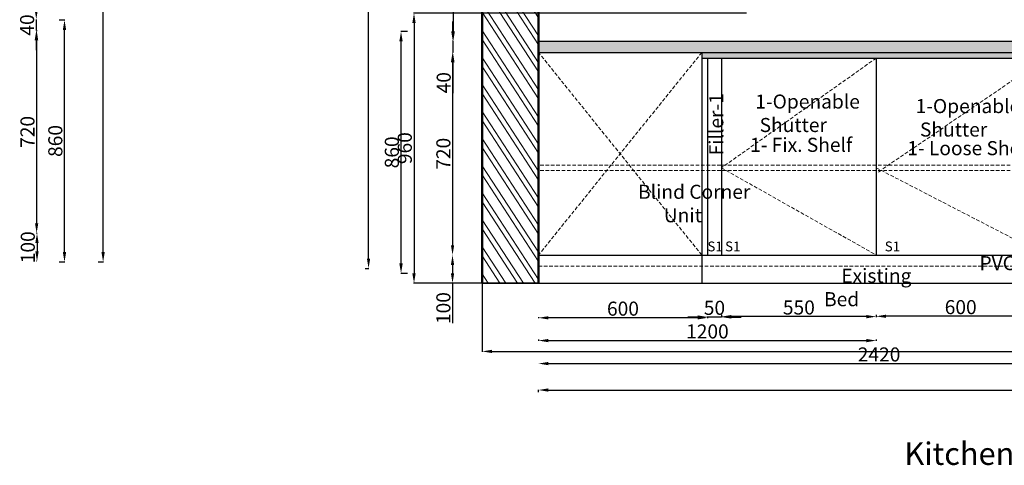
# Model space of a CAD drawing. Units: millimetres. Extents: x 407065 to 421840, y 1168257 to 1177792.
# Tile 15 of 17: x 415758 to 419256, y 1173419 to 1175003. Entities that reach past the tile are written whole.
import ezdxf

# ---------------------------------------------------------------- set-up
doc = ezdxf.new("R2010")
doc.units = ezdxf.units.MM
doc.linetypes.add('DASHED', pattern=[19.05, 12.7, -6.35])
for name, color, linetype, lineweight in [('A-ANNO-DIMS', 6, 'Continuous', 18), ('A-ANNO-TEXT', 30, 'Continuous', 18), ('A-FURN', 3, 'Continuous', 25), ('A-FURN-HIDN', 7, 'DASHED', 18), ('A-FURN-PATT', 252, 'Continuous', 13), ('A-WALL', 7, 'Continuous', 50), ('A-WALL-PATT', 8, 'Continuous', 13)]:
    doc.layers.add(name, color=color, linetype=linetype, lineweight=lineweight)
doc.styles.get("Standard").update_dxf_attribs({"font": 'arial.ttf'})
doc.dimstyles.new('ISO-25', dxfattribs={"dimtxt": 50, "dimasz": 35, "dimexe": 1.25, "dimexo": 0.625, "dimtad": 1, "dimdec": 1, "dimtxsty": 'Standard', "dimcen": 35, "dimadec": 0, "dimazin": 0, "dimtfac": 1, "dimtdec": 1, "dimtmove": 0, "dimatfit": 3, "dimfxl": 1, "dimarcsym": 0})

# ---------------------------------------------------------------- blocks, each defined once
blk = doc.blocks.new('*D67')
at = {"layer": 'A-ANNO-DIMS', "color": 0, "lineweight": -2, "transparency": 16777216}
for p, q in [((415816.7, 1175038.9), (415816.7, 1175073.9)), ((415816.7, 1175003.9), (415816.7, 1174963.9)), ((415817.3, 1175003.9), (415817.9, 1175003.9)), ((415817.3, 1174963.9), (415817.9, 1174963.9)), ((415816.7, 1174928.9), (415816.7, 1174893.9))]:
    blk.add_line(p, q, dxfattribs=at)
at = {"layer": 'A-ANNO-DIMS', "color": 0, "transparency": 16777216}
for points in [[(415810.8, 1175038.9), (415822.5, 1175038.9), (415816.7, 1175003.9)], [(415810.8, 1174928.9), (415822.5, 1174928.9), (415816.7, 1174963.9)]]:
    blk.add_solid(points, dxfattribs=at)
at = {"layer": 'Defpoints', "color": 0, "transparency": 16777216}
for p in [(415816.7, 1175003.9), (415816.7, 1174963.9), (415816.7, 1174963.9)]:
    blk.add_point(p, dxfattribs=at)
at = {"layer": 'A-ANNO-DIMS', "color": 0, "transparency": 16777216, "insert": (415790.5, 1174983.9), "char_height": 50, "attachment_point": 5, "rotation": 90}
blk.add_mtext('40', dxfattribs=at)
blk = doc.blocks.new('*D68')
at = {"layer": 'A-ANNO-DIMS', "color": 0, "lineweight": -2, "transparency": 16777216}
for p, q in [((415817.3, 1174963.9), (415819.2, 1174963.9)), ((415817.9, 1174928.9), (415817.9, 1174278.9)), ((415817.3, 1174243.9), (415819.2, 1174243.9))]:
    blk.add_line(p, q, dxfattribs=at)
at = {"layer": 'A-ANNO-DIMS', "color": 0, "transparency": 16777216}
for points in [[(415812.1, 1174928.9), (415823.7, 1174928.9), (415817.9, 1174963.9)], [(415812.1, 1174278.9), (415823.7, 1174278.9), (415817.9, 1174243.9)]]:
    blk.add_solid(points, dxfattribs=at)
at = {"layer": 'Defpoints', "color": 0, "transparency": 16777216}
for p in [(415816.7, 1174963.9), (415816.7, 1174243.9), (415817.9, 1174243.9)]:
    blk.add_point(p, dxfattribs=at)
at = {"layer": 'A-ANNO-DIMS', "color": 0, "transparency": 16777216, "insert": (415791.8, 1174603.9), "char_height": 50, "attachment_point": 5, "rotation": 90}
blk.add_mtext('720', dxfattribs=at)
blk = doc.blocks.new('*D69')
at = {"layer": 'A-ANNO-DIMS', "color": 0, "lineweight": -2, "transparency": 16777216}
for p, q in [((415818.5, 1174243.9), (415817.9, 1174243.9)), ((415819.2, 1174208.9), (415819.2, 1174178.9)), ((415818.5, 1174143.9), (415817.9, 1174143.9))]:
    blk.add_line(p, q, dxfattribs=at)
at = {"layer": 'A-ANNO-DIMS', "color": 0, "transparency": 16777216}
for points in [[(415813.3, 1174208.9), (415825, 1174208.9), (415819.2, 1174243.9)], [(415813.3, 1174178.9), (415825, 1174178.9), (415819.2, 1174143.9)]]:
    blk.add_solid(points, dxfattribs=at)
at = {"layer": 'Defpoints', "color": 0, "transparency": 16777216}
for p in [(415819.2, 1174243.9), (415819.2, 1174143.9), (415819.2, 1174143.9)]:
    blk.add_point(p, dxfattribs=at)
at = {"layer": 'A-ANNO-DIMS', "color": 0, "transparency": 16777216, "insert": (415793, 1174193.9), "char_height": 50, "attachment_point": 5, "rotation": 90}
blk.add_mtext('100', dxfattribs=at)
blk = doc.blocks.new('*D70')
at = {"layer": 'A-ANNO-DIMS', "color": 0, "lineweight": -2, "transparency": 16777216}
for p, q in [((415898.4, 1175001.7), (415918.2, 1175001.7)), ((415916.9, 1174176.7), (415916.9, 1174966.7)), ((415898.4, 1174141.7), (415918.2, 1174141.7))]:
    blk.add_line(p, q, dxfattribs=at)
at = {"layer": 'A-ANNO-DIMS', "color": 0, "transparency": 16777216}
for points in [[(415911.1, 1174966.7), (415922.8, 1174966.7), (415916.9, 1175001.7)], [(415911.1, 1174176.7), (415922.8, 1174176.7), (415916.9, 1174141.7)]]:
    blk.add_solid(points, dxfattribs=at)
at = {"layer": 'Defpoints', "color": 0, "transparency": 16777216}
for p in [(415897.8, 1175001.7), (415916.9, 1175001.7), (415897.8, 1174141.7)]:
    blk.add_point(p, dxfattribs=at)
at = {"layer": 'A-ANNO-DIMS', "color": 0, "transparency": 16777216, "insert": (415890.8, 1174571.7), "char_height": 50, "attachment_point": 5, "rotation": 90}
blk.add_mtext('860', dxfattribs=at)
blk = doc.blocks.new('*D71')
at = {"layer": 'A-ANNO-DIMS', "color": 0, "lineweight": -2, "transparency": 16777216}
for p, q in [((416036.8, 1176991.7), (416055.3, 1176991.7)), ((416054.1, 1174176.7), (416054.1, 1176956.7)), ((416036.8, 1174141.7), (416055.3, 1174141.7))]:
    blk.add_line(p, q, dxfattribs=at)
at = {"layer": 'A-ANNO-DIMS', "color": 0, "transparency": 16777216}
for points in [[(416048.2, 1176956.7), (416059.9, 1176956.7), (416054.1, 1176991.7)], [(416048.2, 1174176.7), (416059.9, 1174176.7), (416054.1, 1174141.7)]]:
    blk.add_solid(points, dxfattribs=at)
at = {"layer": 'Defpoints', "color": 0, "transparency": 16777216}
for p in [(416036.2, 1176991.7), (416054.1, 1176991.7), (416036.2, 1174141.7)]:
    blk.add_point(p, dxfattribs=at)
at = {"layer": 'A-ANNO-DIMS', "color": 0, "transparency": 16777216, "insert": (416027.9, 1175566.7), "char_height": 50, "attachment_point": 5, "rotation": 90}
blk.add_mtext('2850', dxfattribs=at)
blk = doc.blocks.new('*D97')
at = {"layer": 'A-ANNO-DIMS', "color": 0, "lineweight": -2, "transparency": 16777216}
for p, q in [((418801.3, 1173953.7), (418801.3, 1173947.3)), ((419401.3, 1173953.7), (419401.3, 1173947.3)), ((419366.3, 1173948.5), (418836.3, 1173948.5))]:
    blk.add_line(p, q, dxfattribs=at)
at = {"layer": 'A-ANNO-DIMS', "color": 0, "transparency": 16777216}
for points in [[(418836.3, 1173954.3), (418836.3, 1173942.7), (418801.3, 1173948.5)], [(419366.3, 1173954.3), (419366.3, 1173942.7), (419401.3, 1173948.5)]]:
    blk.add_solid(points, dxfattribs=at)
at = {"layer": 'Defpoints', "color": 0, "transparency": 16777216}
for p in [(418801.3, 1173954.3), (419401.3, 1173954.3), (418801.3, 1173948.5)]:
    blk.add_point(p, dxfattribs=at)
at = {"layer": 'A-ANNO-DIMS', "color": 0, "transparency": 16777216, "insert": (419101.3, 1173974.7), "char_height": 50, "attachment_point": 5}
blk.add_mtext('600', dxfattribs=at)
blk = doc.blocks.new('*D98')
at = {"layer": 'A-ANNO-DIMS', "color": 0, "lineweight": -2, "transparency": 16777216}
for p, q in [((418251.3, 1173953.7), (418251.3, 1173946)), ((418801.3, 1173953.7), (418801.3, 1173946)), ((418766.3, 1173947.3), (418286.3, 1173947.3))]:
    blk.add_line(p, q, dxfattribs=at)
at = {"layer": 'A-ANNO-DIMS', "color": 0, "transparency": 16777216}
for points in [[(418286.3, 1173953.1), (418286.3, 1173941.4), (418251.3, 1173947.3)], [(418766.3, 1173953.1), (418766.3, 1173941.4), (418801.3, 1173947.3)]]:
    blk.add_solid(points, dxfattribs=at)
at = {"layer": 'Defpoints', "color": 0, "transparency": 16777216}
for p in [(418251.3, 1173954.3), (418801.3, 1173954.3), (418251.3, 1173947.3)]:
    blk.add_point(p, dxfattribs=at)
at = {"layer": 'A-ANNO-DIMS', "color": 0, "transparency": 16777216, "insert": (418526.3, 1173973.4), "char_height": 50, "attachment_point": 5}
blk.add_mtext('550', dxfattribs=at)
blk = doc.blocks.new('*D99')
at = {"layer": 'A-ANNO-DIMS', "color": 0, "lineweight": -2, "transparency": 16777216}
for p, q in [((418166.3, 1173946), (418131.3, 1173946)), ((418201.3, 1173946.6), (418201.3, 1173947.3)), ((418251.3, 1173946), (418201.3, 1173946)), ((418251.3, 1173946.6), (418251.3, 1173947.3)), ((418286.3, 1173946), (418321.3, 1173946))]:
    blk.add_line(p, q, dxfattribs=at)
at = {"layer": 'A-ANNO-DIMS', "color": 0, "transparency": 16777216}
for points in [[(418166.3, 1173951.8), (418166.3, 1173940.2), (418201.3, 1173946)], [(418286.3, 1173951.8), (418286.3, 1173940.2), (418251.3, 1173946)]]:
    blk.add_solid(points, dxfattribs=at)
at = {"layer": 'Defpoints', "color": 0, "transparency": 16777216}
for p in [(418201.3, 1173946), (418201.3, 1173946), (418251.3, 1173946)]:
    blk.add_point(p, dxfattribs=at)
at = {"layer": 'A-ANNO-DIMS', "color": 0, "transparency": 16777216, "insert": (418226.3, 1173972.2), "char_height": 50, "attachment_point": 5}
blk.add_mtext('50', dxfattribs=at)
blk = doc.blocks.new('*D100')
at = {"layer": 'A-ANNO-DIMS', "color": 0, "lineweight": -2, "transparency": 16777216}
for p, q in [((417601.3, 1173945.4), (417601.3, 1173941.8)), ((418166.3, 1173943.1), (417636.3, 1173943.1)), ((418201.3, 1173945.4), (418201.3, 1173941.8))]:
    blk.add_line(p, q, dxfattribs=at)
at = {"layer": 'A-ANNO-DIMS', "color": 0, "transparency": 16777216}
for points in [[(417636.3, 1173948.9), (417636.3, 1173937.3), (417601.3, 1173943.1)], [(418166.3, 1173948.9), (418166.3, 1173937.3), (418201.3, 1173943.1)]]:
    blk.add_solid(points, dxfattribs=at)
at = {"layer": 'Defpoints', "color": 0, "transparency": 16777216}
for p in [(417601.3, 1173946), (417601.3, 1173943.1), (418201.3, 1173946)]:
    blk.add_point(p, dxfattribs=at)
at = {"layer": 'A-ANNO-DIMS', "color": 0, "transparency": 16777216, "insert": (417901.3, 1173969.2), "char_height": 50, "attachment_point": 5}
blk.add_mtext('600', dxfattribs=at)
blk = doc.blocks.new('*D101')
at = {"layer": 'A-ANNO-DIMS', "color": 0, "lineweight": -2, "transparency": 16777216}
for p, q in [((417601.3, 1173866.3), (417601.3, 1173860.9)), ((417636.3, 1173862.2), (418766.3, 1173862.2)), ((418801.3, 1173866.3), (418801.3, 1173860.9))]:
    blk.add_line(p, q, dxfattribs=at)
at = {"layer": 'A-ANNO-DIMS', "color": 0, "transparency": 16777216}
for points in [[(417636.3, 1173868), (417636.3, 1173856.3), (417601.3, 1173862.2)], [(418766.3, 1173868), (418766.3, 1173856.3), (418801.3, 1173862.2)]]:
    blk.add_solid(points, dxfattribs=at)
at = {"layer": 'Defpoints', "color": 0, "transparency": 16777216}
for p in [(417601.3, 1173867), (418801.3, 1173867), (418801.3, 1173862.2)]:
    blk.add_point(p, dxfattribs=at)
at = {"layer": 'A-ANNO-DIMS', "color": 0, "transparency": 16777216, "insert": (418201.3, 1173888.3), "char_height": 50, "attachment_point": 5}
blk.add_mtext('1200', dxfattribs=at)
blk = doc.blocks.new('*D102')
at = {"layer": 'A-ANNO-DIMS', "color": 0, "lineweight": -2, "transparency": 16777216}
for p, q in [((417601.3, 1173779.7), (417601.3, 1173779.1)), ((417636.3, 1173780.4), (419986.3, 1173780.4)), ((420021.3, 1173779.7), (420021.3, 1173779.1))]:
    blk.add_line(p, q, dxfattribs=at)
at = {"layer": 'A-ANNO-DIMS', "color": 0, "transparency": 16777216}
for points in [[(417636.3, 1173786.2), (417636.3, 1173774.5), (417601.3, 1173780.4)], [(419986.3, 1173786.2), (419986.3, 1173774.5), (420021.3, 1173780.4)]]:
    blk.add_solid(points, dxfattribs=at)
at = {"layer": 'Defpoints', "color": 0, "transparency": 16777216}
for p in [(417601.3, 1173780.4), (420021.3, 1173780.4), (420021.3, 1173780.4)]:
    blk.add_point(p, dxfattribs=at)
at = {"layer": 'A-ANNO-DIMS', "color": 0, "transparency": 16777216, "insert": (418811.3, 1173806.5), "char_height": 50, "attachment_point": 5}
blk.add_mtext('2420', dxfattribs=at)
blk = doc.blocks.new('*D103')
at = {"layer": 'A-ANNO-DIMS', "color": 0, "lineweight": -2, "transparency": 16777216}
for p, q in [((417601.3, 1173679.4), (417601.3, 1173687.7)), ((417636.3, 1173686.5), (421356.3, 1173686.5)), ((421391.3, 1173679.4), (421391.3, 1173687.7))]:
    blk.add_line(p, q, dxfattribs=at)
at = {"layer": 'A-ANNO-DIMS', "color": 0, "transparency": 16777216}
for points in [[(417636.3, 1173692.3), (417636.3, 1173680.6), (417601.3, 1173686.5)], [(421356.3, 1173692.3), (421356.3, 1173680.6), (421391.3, 1173686.5)]]:
    blk.add_solid(points, dxfattribs=at)
at = {"layer": 'Defpoints', "color": 0, "transparency": 16777216}
for p in [(417601.3, 1173678.8), (421391.3, 1173686.5), (421391.3, 1173678.8)]:
    blk.add_point(p, dxfattribs=at)
at = {"layer": 'A-ANNO-DIMS', "color": 0, "transparency": 16777216, "insert": (419496.3, 1173712.6), "char_height": 50, "attachment_point": 5}
blk.add_mtext('3790', dxfattribs=at)
blk = doc.blocks.new('*D107')
at = {"layer": 'A-ANNO-DIMS', "color": 0, "lineweight": -2, "transparency": 16777216}
for p, q in [((417298.8, 1175526.2), (417299.5, 1175526.2)), ((417298.2, 1175491.2), (417298.2, 1174961.2)), ((417298.8, 1174926.2), (417299.5, 1174926.2))]:
    blk.add_line(p, q, dxfattribs=at)
at = {"layer": 'A-ANNO-DIMS', "color": 0, "transparency": 16777216}
for points in [[(417292.4, 1175491.2), (417304, 1175491.2), (417298.2, 1175526.2)], [(417292.4, 1174961.2), (417304, 1174961.2), (417298.2, 1174926.2)]]:
    blk.add_solid(points, dxfattribs=at)
at = {"layer": 'Defpoints', "color": 0, "transparency": 16777216}
for p in [(417298.2, 1175526.2), (417298.2, 1174926.2), (417298.2, 1174926.2)]:
    blk.add_point(p, dxfattribs=at)
at = {"layer": 'A-ANNO-DIMS', "color": 0, "transparency": 16777216, "insert": (417272.1, 1175226.2), "char_height": 50, "attachment_point": 5, "rotation": 90}
blk.add_mtext('600', dxfattribs=at)
blk = doc.blocks.new('*D108')
at = {"layer": 'A-ANNO-DIMS', "color": 0, "lineweight": -2, "transparency": 16777216}
for p, q in [((417297, 1174961.2), (417297, 1174996.2)), ((417297.6, 1174926.2), (417295.7, 1174926.2)), ((417297, 1174926.2), (417297, 1174886.2)), ((417297.6, 1174886.2), (417295.7, 1174886.2)), ((417297, 1174851.2), (417297, 1174741.5))]:
    blk.add_line(p, q, dxfattribs=at)
at = {"layer": 'A-ANNO-DIMS', "color": 0, "transparency": 16777216}
for points in [[(417291.1, 1174961.2), (417302.8, 1174961.2), (417297, 1174926.2)], [(417291.1, 1174851.2), (417302.8, 1174851.2), (417297, 1174886.2)]]:
    blk.add_solid(points, dxfattribs=at)
at = {"layer": 'Defpoints', "color": 0, "transparency": 16777216}
for p in [(417298.2, 1174926.2), (417297, 1174886.2), (417298.2, 1174886.2)]:
    blk.add_point(p, dxfattribs=at)
at = {"layer": 'A-ANNO-DIMS', "color": 0, "transparency": 16777216, "insert": (417270.8, 1174778.8), "char_height": 50, "attachment_point": 5, "rotation": 90}
blk.add_mtext('40', dxfattribs=at)
blk = doc.blocks.new('*D109')
at = {"layer": 'A-ANNO-DIMS', "color": 0, "lineweight": -2, "transparency": 16777216}
for p, q in [((417296.3, 1174886.2), (417297, 1174886.2)), ((417295.7, 1174851.2), (417295.7, 1174201.2)), ((417296.3, 1174166.2), (417297, 1174166.2))]:
    blk.add_line(p, q, dxfattribs=at)
at = {"layer": 'A-ANNO-DIMS', "color": 0, "transparency": 16777216}
for points in [[(417289.9, 1174851.2), (417301.5, 1174851.2), (417295.7, 1174886.2)], [(417289.9, 1174201.2), (417301.5, 1174201.2), (417295.7, 1174166.2)]]:
    blk.add_solid(points, dxfattribs=at)
at = {"layer": 'Defpoints', "color": 0, "transparency": 16777216}
for p in [(417295.7, 1174886.2), (417295.7, 1174166.2), (417295.7, 1174166.2)]:
    blk.add_point(p, dxfattribs=at)
at = {"layer": 'A-ANNO-DIMS', "color": 0, "transparency": 16777216, "insert": (417269.6, 1174526.2), "char_height": 50, "attachment_point": 5, "rotation": 90}
blk.add_mtext('720', dxfattribs=at)
blk = doc.blocks.new('*D110')
at = {"layer": 'A-ANNO-DIMS', "color": 0, "lineweight": -2, "transparency": 16777216}
for p, q in [((417296.3, 1174166.2), (417297, 1174166.2)), ((417295.7, 1174131.2), (417295.7, 1174101.2)), ((417295.7, 1174066.2), (417295.7, 1173924.3)), ((417296.3, 1174066.2), (417297, 1174066.2))]:
    blk.add_line(p, q, dxfattribs=at)
at = {"layer": 'A-ANNO-DIMS', "color": 0, "transparency": 16777216}
for points in [[(417289.9, 1174131.2), (417301.5, 1174131.2), (417295.7, 1174166.2)], [(417289.9, 1174101.2), (417301.5, 1174101.2), (417295.7, 1174066.2)]]:
    blk.add_solid(points, dxfattribs=at)
at = {"layer": 'Defpoints', "color": 0, "transparency": 16777216}
for p in [(417295.7, 1174166.2), (417295.7, 1174066.2), (417295.7, 1174066.2)]:
    blk.add_point(p, dxfattribs=at)
at = {"layer": 'A-ANNO-DIMS', "color": 0, "transparency": 16777216, "insert": (417269.6, 1173977.7), "char_height": 50, "attachment_point": 5, "rotation": 90}
blk.add_mtext('100', dxfattribs=at)
blk = doc.blocks.new('*D111')
at = {"layer": 'A-ANNO-DIMS', "color": 0, "lineweight": -2, "transparency": 16777216}
for p, q in [((417135.1, 1174961.2), (417111.4, 1174961.2)), ((417112.7, 1174136.2), (417112.7, 1174926.2)), ((417135.1, 1174101.2), (417111.4, 1174101.2))]:
    blk.add_line(p, q, dxfattribs=at)
at = {"layer": 'A-ANNO-DIMS', "color": 0, "transparency": 16777216}
for points in [[(417106.8, 1174926.2), (417118.5, 1174926.2), (417112.7, 1174961.2)], [(417106.8, 1174136.2), (417118.5, 1174136.2), (417112.7, 1174101.2)]]:
    blk.add_solid(points, dxfattribs=at)
at = {"layer": 'Defpoints', "color": 0, "transparency": 16777216}
for p in [(417112.7, 1174961.2), (417135.8, 1174961.2), (417135.8, 1174101.2)]:
    blk.add_point(p, dxfattribs=at)
at = {"layer": 'A-ANNO-DIMS', "color": 0, "transparency": 16777216, "insert": (417086.5, 1174531.2), "char_height": 50, "attachment_point": 5, "rotation": 90}
blk.add_mtext('860', dxfattribs=at)
blk = doc.blocks.new('*D112')
at = {"layer": 'A-ANNO-DIMS', "color": 0, "lineweight": -2, "transparency": 16777216}
for p, q in [((416985.7, 1176968.7), (416998.5, 1176968.7)), ((416997.3, 1174153.7), (416997.3, 1176933.7)), ((416985.7, 1174118.7), (416998.5, 1174118.7))]:
    blk.add_line(p, q, dxfattribs=at)
at = {"layer": 'A-ANNO-DIMS', "color": 0, "transparency": 16777216}
for points in [[(416991.4, 1176933.7), (417003.1, 1176933.7), (416997.3, 1176968.7)], [(416991.4, 1174153.7), (417003.1, 1174153.7), (416997.3, 1174118.7)]]:
    blk.add_solid(points, dxfattribs=at)
at = {"layer": 'Defpoints', "color": 0, "transparency": 16777216}
for p in [(416985.1, 1176968.7), (416997.3, 1176968.7), (416985.1, 1174118.7)]:
    blk.add_point(p, dxfattribs=at)
at = {"layer": 'A-ANNO-DIMS', "color": 0, "transparency": 16777216, "insert": (416971.1, 1175543.7), "char_height": 50, "attachment_point": 5, "rotation": 90}
blk.add_mtext('2850', dxfattribs=at)
blk = doc.blocks.new('*D200')
at = {"layer": 'A-ANNO-DIMS', "color": 0, "lineweight": -2, "transparency": 16777216}
for p, q in [((417401.3, 1174065.5), (417401.3, 1173822.4)), ((421591.3, 1174065.5), (421591.3, 1173822.4)), ((417436.3, 1173823.7), (421556.3, 1173823.7))]:
    blk.add_line(p, q, dxfattribs=at)
at = {"layer": 'A-ANNO-DIMS', "color": 0, "transparency": 16777216}
for points in [[(417436.3, 1173829.5), (417436.3, 1173817.8), (417401.3, 1173823.7)], [(421556.3, 1173829.5), (421556.3, 1173817.8), (421591.3, 1173823.7)]]:
    blk.add_solid(points, dxfattribs=at)
at = {"layer": 'Defpoints', "color": 0, "transparency": 16777216}
for p in [(417401.3, 1174066.2), (421591.3, 1174066.2), (421591.3, 1173823.7)]:
    blk.add_point(p, dxfattribs=at)
at = {"layer": 'A-ANNO-DIMS', "color": 0, "transparency": 16777216, "insert": (419496.3, 1173849.8), "char_height": 50, "attachment_point": 5}
blk.add_mtext('4190', dxfattribs=at)
blk = doc.blocks.new('*D203')
at = {"layer": 'A-ANNO-DIMS', "color": 0, "lineweight": -2, "transparency": 16777216}
for p, q in [((418340.7, 1175026.2), (417157.5, 1175026.2)), ((417158.8, 1174991.2), (417158.8, 1174101.2)), ((417600.7, 1174066.2), (417157.5, 1174066.2))]:
    blk.add_line(p, q, dxfattribs=at)
at = {"layer": 'A-ANNO-DIMS', "color": 0, "transparency": 16777216}
for points in [[(417152.9, 1174991.2), (417164.6, 1174991.2), (417158.8, 1175026.2)], [(417152.9, 1174101.2), (417164.6, 1174101.2), (417158.8, 1174066.2)]]:
    blk.add_solid(points, dxfattribs=at)
at = {"layer": 'Defpoints', "color": 0, "transparency": 16777216}
for p in [(418341.3, 1175026.2), (417158.8, 1174066.2), (417601.3, 1174066.2)]:
    blk.add_point(p, dxfattribs=at)
at = {"layer": 'A-ANNO-DIMS', "color": 0, "transparency": 16777216, "insert": (417132.6, 1174546.2), "char_height": 50, "attachment_point": 5, "rotation": 90}
blk.add_mtext('960', dxfattribs=at)

msp = doc.modelspace()

# ---------------------------------------------------------------- hatches: boundary and pattern name
at = {"layer": 'A-FURN-PATT'}
h = msp.add_hatch(dxfattribs=at)
h.set_pattern_fill('AR-CONC', color=256, scale=0.08)
h.set_pattern_definition([(50, (-3404.924, -221.627), (14.57477352, -1.27512684), [1.524, -16.764]), (355, (-3404.924, -221.627), (-2.81947371, 15.28454762), [1.2192, -13.41124673]), (100.4514447, (-3403.709, -221.733), (11.75529977, 14.00942015), [1.2952007, -14.24721957]), (46.1842, (-3404.924, -217.563), (21.68632327, -3.36338623), [2.286, -25.146]), (96.6355576, (-3403.116, -217.843), (18.99233072, 19.79408997), [1.94280185, -21.37084865]), (351.1841512, (-3404.924, -217.563), (18.99233073, 19.79408997), [1.82879737, -20.11677855]), (21, (-3402.892, -218.579), (12.1291513, -8.18121585), [1.524, -16.764]), (326, (-3402.892, -218.579), (4.94416227, 14.73503729), [1.2192, -13.4112]), (71.451445, (-3401.881, -219.261), (17.07331354, 6.55382151), [1.2952007, -14.247195]), (37.5, (-3404.9237, -221.627), (0.24708826, 6.76440311), [0, -13.24864, 0, -13.6144, 0, -13.462]), (7.5, (-3404.924, -221.627), (5.345573, 8.014445985), [0, -7.76224, 0, -12.94384, 0, -5.1308]), (327.5, (-3409.455, -221.627), (10.847247613, -0.45829952), [0, -5.08, 0, -15.8496, 0, -21.0312]), (317.5, (-3411.487, -221.627), (11.85033451, 2.03411928), [0, -6.604, 0, -10.52576, 0, -14.9352])])
h.paths.add_polyline_path([(420021.277, 1174926.1682), (417601.277, 1174926.1682), (417601.277, 1174886.1682), (420021.277, 1174886.1682)])
h = msp.add_hatch(color=256, dxfattribs=at)
h.dxf.hatch_style = 1
h.paths.add_polyline_path([(420001.277, 1174886.1682), (418181.277, 1174886.1682), (418181.277, 1174866.1682), (420001.277, 1174866.1682)])
at = {"layer": 'A-WALL-PATT'}
h = msp.add_hatch(dxfattribs=at)
h.set_pattern_fill('ANSI32', color=256, scale=5.5, angle=78)
h.set_pattern_definition([(123, (-3404.924, -221.627), (-43.9358544, -28.5322774), []), (123, (-3399.79, -197.47), (-43.9358544, -28.5322774), [])])
h.paths.add_polyline_path([(417601.277, 1176916.1682), (417401.277, 1176916.1682), (417401.277, 1174066.1682), (417601.277, 1174066.1682)])

# ---------------------------------------------------------------- linework, layer by layer
at = {"layer": 'A-FURN'}
for p, q in [((417601.277, 1174926.1682), (420021.277, 1174926.1682)), ((417601.277, 1174886.1682), (420021.277, 1174886.1682)), ((418181.277, 1174866.1682), (420001.277, 1174866.1682)), ((417601.277, 1174166.1682), (420001.277, 1174166.1682)), ((417401.277, 1174066.1682), (421591.277, 1174066.1682))]:
    msp.add_line(p, q, dxfattribs=at)
for points in [[(418181.277, 1174886.1682), (418181.277, 1174066.1682)], [(418201.277, 1174866.1682), (418201.277, 1174166.1682)], [(418251.277, 1174866.1682), (418251.277, 1174166.1682)], [(418801.277, 1174866.1682), (418801.277, 1174166.1682)]]:
    msp.add_lwpolyline(points, dxfattribs=at)
at = {"layer": 'A-FURN-HIDN'}
for p, q in [((418181.277, 1174886.1682), (417601.277, 1174166.1682)), ((418181.277, 1174166.1682), (417601.277, 1174886.1682)), ((418801.277, 1174866.1682), (418251.277, 1174476.1682)), ((419401.277, 1174866.1682), (418801.277, 1174456.1682)), ((420001.277, 1174486.1682), (417601.277, 1174486.1682)), ((418251.277, 1174476.1682), (418801.277, 1174166.1682)), ((418801.277, 1174476.1682), (419401.277, 1174166.1682)), ((420001.277, 1174466.1682), (417601.277, 1174466.1682)), ((417601.277, 1174126.1682), (421391.277, 1174126.1682))]:
    msp.add_line(p, q, dxfattribs=at)
at = {"layer": 'A-WALL'}
for p, q in [((417401.277, 1176916.1682), (417401.277, 1174066.1682)), ((417601.277, 1176916.1682), (417601.277, 1174066.1682))]:
    msp.add_line(p, q, dxfattribs=at)

# ---------------------------------------------------------------- texts
at = {"layer": 'A-ANNO-TEXT', "insert": (418207.8077, 1174444.1465), "char_height": 50, "attachment_point": 1, "rotation": 90}
msp.add_mtext_dynamic_manual_height_columns('     Filler-1', width=382.409863, gutter_width=12.5, heights=[0], dxfattribs=at)
at = {"layer": 'A-ANNO-TEXT', "attachment_point": 1}
for s, width, insert, char_height in [('     1-Openable\\P      Shutter', 520.083559, (418295.1181, 1174736.8142), 50), ('     1-Openable\\P      Shutter', 520.083559, (418864.8173, 1174720.715), 50), ('1- Fix. Shelf', 382.409863, (418353.0836, 1174582.9414), 50), ('\\pxt7;1- Loose Shelf', 487.590713, (418911.573, 1174571.1227), 50), ('Blind Corner\\P      Unit', 632.856839, (417954.8072, 1174416.0282), 50), ('S1', 382.409863, (418201.277, 1174214.2734), 35), ('S1', 382.409863, (418263.9785, 1174214.2734), 35), ('S1', 382.409863, (418831.3476, 1174214.2734), 35), ('    PVC Skirting', 640.76562, (419106.9011, 1174162.362), 50), ('    Existing Bed', 382.409863, (418615.7966, 1174117.6632), 50), ('Kitchen Elevation At-B', 1357.183536, (418901.2019, 1173500.2608), 80)]:
    msp.add_mtext_dynamic_manual_height_columns(s, width=width, gutter_width=12.5, heights=[0], dxfattribs=dict(at, insert=insert, char_height=char_height))

# ---------------------------------------------------------------- dimensions: what is measured, and where the dimension line sits
at = {"layer": 'A-ANNO-DIMS'}
for base, p1, p2, override, picture, middle in [((416054.0818, 1176991.6535), (416036.1552, 1174141.6535), (416036.1552, 1176991.6535), {"dimclrd": 0, "dimclre": 0, "dimclrt": 0}, '*D71', (416027.9281, 1175566.6535)), ((416997.263, 1176968.6682), (416985.074, 1174118.6682), (416985.074, 1176968.6682), {"dimclrd": 0, "dimclre": 0, "dimclrt": 0}, '*D112', (416971.1094, 1175543.6682)), ((417298.2094, 1174926.1682), (417298.2094, 1175526.1682), (417298.2094, 1174926.1682), {"dimclrd": 0, "dimclre": 0, "dimclrt": 0}, '*D107', (417272.0557, 1175226.1682)), ((415916.9498, 1175001.6535), (415897.8122, 1174141.6535), (415897.8122, 1175001.6535), {"dimclrd": 0, "dimclre": 0, "dimclrt": 0}, '*D70', (415890.7962, 1174571.6535)), ((417158.777, 1174066.1682), (418341.277, 1175026.1682), (417601.277, 1174066.1682), {"dimdec": 0, "dimlfac": 1, "dimrnd": 0, "dimzin": 0, "dimdsep": 46, "dimlunit": 2}, '*D203', (417132.6234, 1174546.1682)), ((417296.9594, 1174886.1682), (417298.2094, 1174926.1682), (417298.2094, 1174886.1682), {"dimclrd": 0, "dimclre": 0, "dimclrt": 0}, '*D108', (417270.8057, 1174778.8106)), ((415817.9041, 1174243.913), (415816.6541, 1174963.913), (415816.6541, 1174243.913), {"dimclrd": 0, "dimclre": 0, "dimclrt": 0}, '*D68', (415791.7505, 1174603.913)), ((417112.6678, 1174961.1682), (417135.7568, 1174101.1682), (417135.7568, 1174961.1682), {"dimclrd": 0, "dimclre": 0, "dimclrt": 0}, '*D111', (417086.5142, 1174531.1682)), ((417295.7094, 1174166.1682), (417295.7094, 1174886.1682), (417295.7094, 1174166.1682), {"dimclrd": 0, "dimclre": 0, "dimclrt": 0}, '*D109', (417269.5557, 1174526.1682)), ((417295.7094, 1174066.1682), (417295.7094, 1174166.1682), (417295.7094, 1174066.1682), {"dimclrd": 0, "dimclre": 0, "dimclrt": 0}, '*D110', (417269.5557, 1173977.7465))]:
    dim = msp.add_linear_dim(base=base, p1=p1, p2=p2, angle=90, dimstyle='ISO-25', override=override, dxfattribs=at)
    dim.commit()
    dim.dimension.update_dxf_attribs({"geometry": picture, "text_midpoint": middle})
for base, p1, p2, picture, middle in [((415816.6541, 1174963.913), (415816.6541, 1175003.913), (415816.6541, 1174963.913), '*D67', (415816.6541, 1174983.913)), ((415819.1541, 1174143.913), (415819.1541, 1174243.913), (415819.1541, 1174143.913), '*D69', (415819.1541, 1174193.913))]:
    dim = msp.add_linear_dim(base=base, p1=p1, p2=p2, angle=90, dimstyle='ISO-25', override={"dimclrd": 0, "dimclre": 0, "dimclrt": 0}, dxfattribs=at)
    dim.commit()
    dim.dimension.update_dxf_attribs({"geometry": picture, "text_midpoint": middle, "dimtype": 160})
for base, p1, p2, override, picture, middle in [((421591.277, 1173823.6682), (417401.277, 1174066.1682), (421591.277, 1174066.1682), {"dimdec": 0, "dimlfac": 1, "dimrnd": 0, "dimzin": 0, "dimdsep": 46, "dimlunit": 2}, '*D200', (419496.277, 1173849.8219)), ((417601.277, 1173943.0963), (418201.277, 1173946.013), (417601.277, 1173946.013), {"dimclrd": 0, "dimclre": 0, "dimclrt": 0}, '*D100', (417901.277, 1173969.25)), ((418251.277, 1173947.263), (418801.277, 1173954.3463), (418251.277, 1173954.3463), {"dimclrd": 0, "dimclre": 0, "dimclrt": 0}, '*D98', (418526.277, 1173973.4166)), ((418801.277, 1173948.513), (419401.277, 1173954.3463), (418801.277, 1173954.3463), {"dimclrd": 0, "dimclre": 0, "dimclrt": 0}, '*D97', (419101.277, 1173974.6666)), ((418801.277, 1173862.1694), (417601.277, 1173866.9579), (418801.277, 1173866.9579), {"dimclrd": 0, "dimclre": 0, "dimclrt": 0}, '*D101', (418201.277, 1173888.323)), ((420021.277, 1173780.3642), (417601.277, 1173780.3668), (420021.277, 1173780.3668), {"dimclrd": 0, "dimclre": 0, "dimclrt": 0}, '*D102', (418811.277, 1173806.5178)), ((421391.277, 1173686.4606), (417601.277, 1173678.7822), (421391.277, 1173678.7822), {"dimclrd": 0, "dimclre": 0, "dimclrt": 0}, '*D103', (419496.277, 1173712.6313))]:
    dim = msp.add_linear_dim(base=base, p1=p1, p2=p2, dimstyle='ISO-25', override=override, dxfattribs=at)
    dim.commit()
    dim.dimension.update_dxf_attribs({"geometry": picture, "text_midpoint": middle})
dim = msp.add_linear_dim(base=(418201.277, 1173946.013), p1=(418251.277, 1173946.013), p2=(418201.277, 1173946.013), dimstyle='ISO-25', override={"dimclrd": 0, "dimclre": 0, "dimclrt": 0}, dxfattribs=at)
dim.commit()
dim.dimension.update_dxf_attribs({"geometry": '*D99', "text_midpoint": (418226.277, 1173946.013), "dimtype": 160})

doc.saveas('drawing.dxf')
